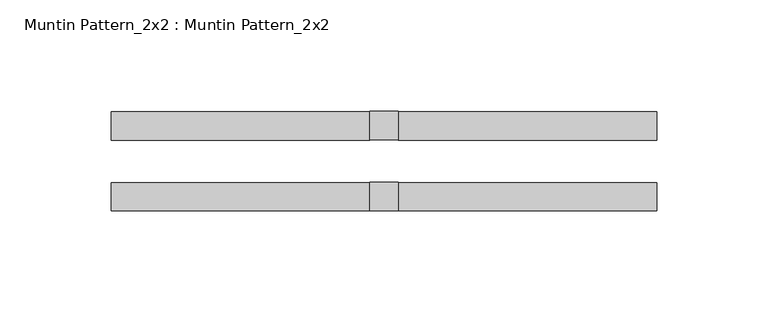
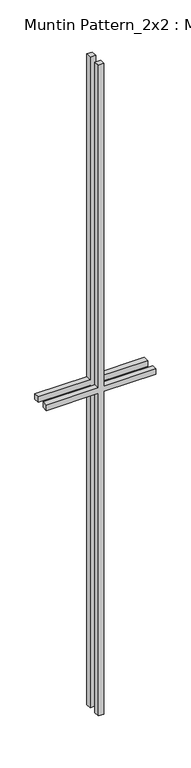
"""IFC4 building model written with IfcOpenShell, lengths in millimetres: proxy geometry, Muntin Pattern_2x2 : Muntin Pattern_2x2."""

from ifc_helpers import new_model, si_unit, frame, origin, place, context, project, spatial, polyline, outline, extrude, source, transform, mapped, element, save


def muntin_pattern_2x2_muntin_pattern_2x2_88561ff7(model_context):
    return source(origin(), model_context, "Body", "SweptSolid", [
        extrude(outline(polyline([(774.7, -6.35), (774.7, -122.2375), (762.0, -122.2375), (762.0, -6.35), (0.0, -6.35), (0.0, 6.35), (762.0, 6.35), (762.0, 122.2375), (774.7, 122.2375), (774.7, 6.35), (1536.7, 6.35), (1536.7, -6.35), (774.7, -6.35)])), frame((0.0, -22.225, 0.0), z_axis=(0.0, 1.0, 0.0), x_axis=(0.0, 0.0, 1.0)), (0.0, 0.0, 1.0), 12.7),
        extrude(outline(polyline([(774.7, -6.35), (774.7, -122.2375), (762.0, -122.2375), (762.0, -6.35), (0.0, -6.35), (0.0, 6.35), (762.0, 6.35), (762.0, 122.2375), (774.7, 122.2375), (774.7, 6.35), (1536.7, 6.35), (1536.7, -6.35), (774.7, -6.35)])), frame((0.0, 9.525, 0.0), z_axis=(0.0, 1.0, 0.0), x_axis=(0.0, 0.0, 1.0)), (0.0, 0.0, 1.0), 12.7),
    ])


if __name__ == "__main__":
    model = new_model("IFC4")
    model_context = context("Model", 3, world=origin())
    ifc_project = project(units=[si_unit("LENGTHUNIT", "METRE", prefix="MILLI")], contexts=[model_context])
    site = spatial("IfcSite", under=ifc_project)
    building = spatial("IfcBuilding", under=site)
    placement = place(None, origin())
    muntin_pattern_2x2_muntin_pattern_2x2_shape = muntin_pattern_2x2_muntin_pattern_2x2_88561ff7(model_context)
    element("IfcBuildingElementProxy", 1, Name="Muntin Pattern_2x2 : Muntin Pattern_2x2", ObjectType="Muntin Pattern_2x2 : Muntin Pattern_2x2", at=placement, inside=building, context=model_context, shape_type="MappedRepresentation", body=[
        mapped(muntin_pattern_2x2_muntin_pattern_2x2_shape, transform((0.0, 0.0, 0.0), x_axis=(1.0, 0.0, 0.0), y_axis=(0.0, 1.0, 0.0), z_axis=(0.0, 0.0, 1.0))),
    ])
    save(model, "model.ifc")

# Revit data of these elements
# Type "Muntin Pattern_2x2 : Muntin Pattern_2x2"
#   Width [instance default] = 4' - 0"
#   Thickness = 0' - 0 1/2"
#   Height [instance default] = 4' - 0"
#   Distance = 0' - 0 3/4"
#   Interior Material [instance default] = none
#   Exterior Material [instance default] = none
#   Default Elevation = 0
# Element 1 (IfcBuildingElementProxy, "Muntin Pattern_2x2 : Muntin Pattern_2x2")
#   Width = 0' - 9 5/8"
#   Height = 5' - 0 1/2"
#   Interior Material = Wood - Stained
#   Exterior Material = Clad - White
#   Materials on its faces: "Clad - White", "Wood - Stained"
# Materials
#   "Clad - White": class "Wood", colour RGB 242 242 238, transparency 0, Cost = 0
#   "Wood - Stained": class "Wood", colour RGB 224 178 126, transparency 0, Cost = 0
